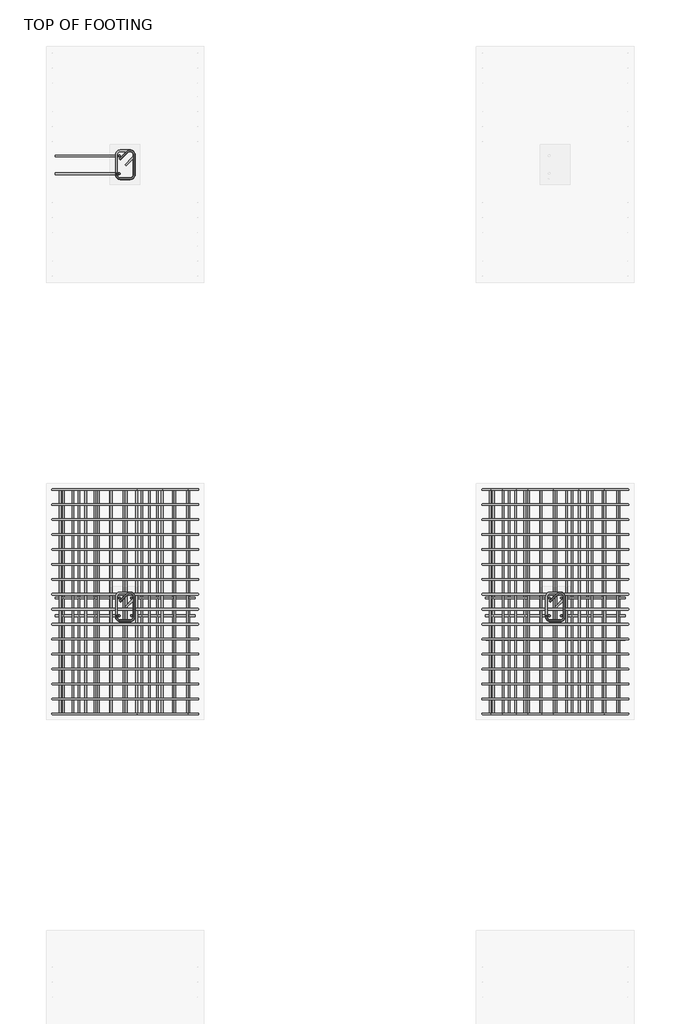
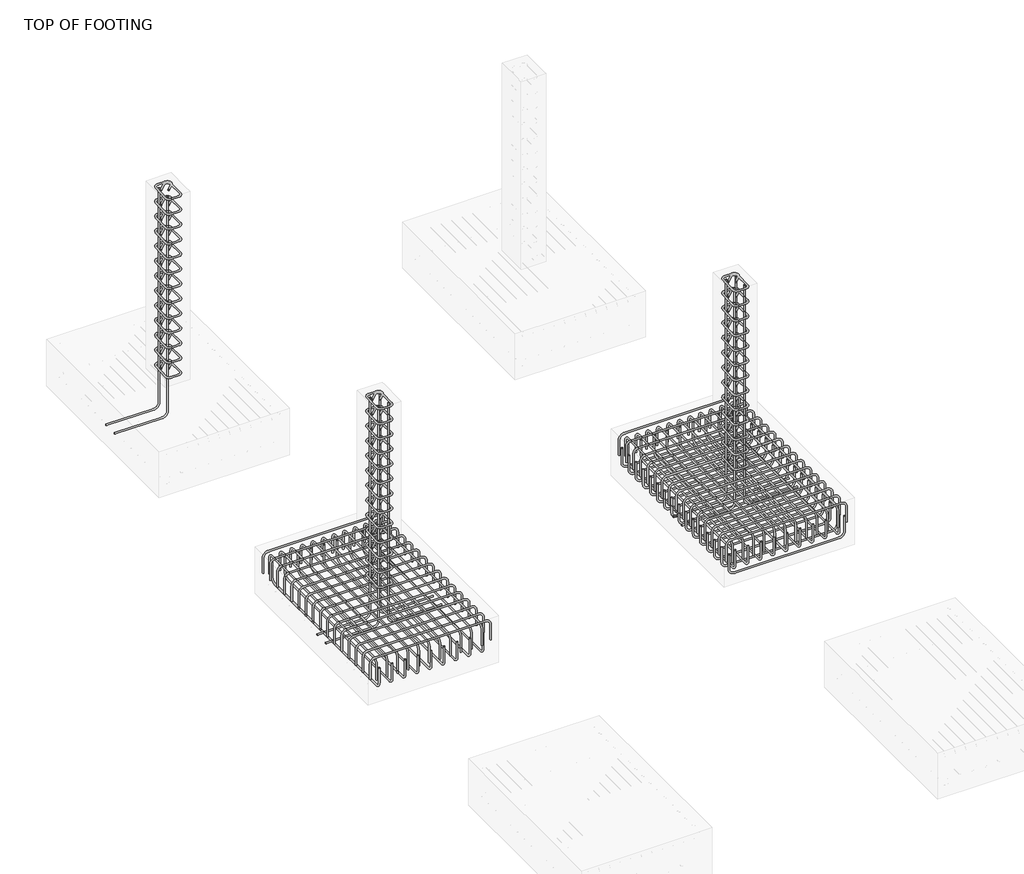
# One storey, part 3 of 8: 15 reinforcing bars.
"""IFC4 building model written with IfcOpenShell, lengths in millimetres."""

from ifc_helpers import new_model, si_unit, point, frame, origin, place, context, project, spatial, polyline, circle_curve, trimmed, segment, composite_curve, source, transform, mapped, element, save
from ifc_brep_helpers import swept_disk

model = new_model("IFC4")

# Units and contexts
model_context = context("Model", 3, world=origin())
ifc_project = project(units=[si_unit("LENGTHUNIT", "METRE", prefix="MILLI")], contexts=[model_context])

# Site, building, storey
site = spatial("IfcSite", under=ifc_project)
building = spatial("IfcBuilding", under=site)
storey = spatial("IfcBuildingStorey", under=building, Name="TOP OF FOOTING", Elevation=-1828.8)

# Reinforcing bars
placement = place(None, origin())
reinforcing_bar_shape = source(origin(), model_context, "Body", "SolidModel", [
    swept_disk(composite_curve([segment(polyline([(-5782.0568817, 6451.7662126, -2068.8), (-5782.0568817, 6451.7662126, -1921.5)]), True, "CONTINUOUS"), segment(trimmed(circle_curve(frame((-5735.7068817, 6451.7662126, -1921.5), z_axis=(0.0, 1.0, 0.0), x_axis=(-46.350000000000364, 0.0, 0.0)), 46.35), [point((-5782.0568817, 6451.7662126, -1921.5))], [point((-5735.7068817, 6451.7662126, -1875.15))], True, "CARTESIAN"), True, "CONTINUOUS"), segment(polyline([(-5735.7068817, 6451.7662126, -1875.15), (-4721.1068817, 6451.7662126, -1875.15)]), True, "CONTINUOUS"), segment(trimmed(circle_curve(frame((-4721.1068817, 6451.7662126, -1921.5), z_axis=(0.0, 1.0, 0.0), x_axis=(0.0, 0.0, 46.34999999999991)), 46.35), [point((-4721.1068817, 6451.7662126, -1875.15))], [point((-4674.7568817, 6451.7662126, -1921.5))], True, "CARTESIAN"), True, "CONTINUOUS"), segment(polyline([(-4674.7568817, 6451.7662126, -1921.5), (-4674.7568817, 6451.7662126, -2068.8)]), True, "CONTINUOUS")], self_intersect=False), 6.35),
])
element("IfcReinforcingBar", 1, at=placement, inside=storey, context=model_context, shape_type="MappedRepresentation", body=[
    mapped(reinforcing_bar_shape, transform((0.0, 0.0, 0.0), x_axis=(1.0, 0.0, 0.0), y_axis=(0.0, 1.0, 0.0), z_axis=(0.0, 0.0, 1.0))),
    mapped(reinforcing_bar_shape, transform((0.0, -113.82, 0.0), x_axis=(1.0, 0.0, 0.0), y_axis=(0.0, 1.0, 0.0), z_axis=(0.0, 0.0, 1.0))),
    mapped(reinforcing_bar_shape, transform((0.0, -227.64, 0.0), x_axis=(1.0, 0.0, 0.0), y_axis=(0.0, 1.0, 0.0), z_axis=(0.0, 0.0, 1.0))),
    mapped(reinforcing_bar_shape, transform((0.0, -341.46, 0.0), x_axis=(1.0, 0.0, 0.0), y_axis=(0.0, 1.0, 0.0), z_axis=(0.0, 0.0, 1.0))),
    mapped(reinforcing_bar_shape, transform((0.0, -455.28, 0.0), x_axis=(1.0, 0.0, 0.0), y_axis=(0.0, 1.0, 0.0), z_axis=(0.0, 0.0, 1.0))),
    mapped(reinforcing_bar_shape, transform((0.0, -569.1, 0.0), x_axis=(1.0, 0.0, 0.0), y_axis=(0.0, 1.0, 0.0), z_axis=(0.0, 0.0, 1.0))),
    mapped(reinforcing_bar_shape, transform((0.0, -682.92, 0.0), x_axis=(1.0, 0.0, 0.0), y_axis=(0.0, 1.0, 0.0), z_axis=(0.0, 0.0, 1.0))),
    mapped(reinforcing_bar_shape, transform((0.0, -796.74, 0.0), x_axis=(1.0, 0.0, 0.0), y_axis=(0.0, 1.0, 0.0), z_axis=(0.0, 0.0, 1.0))),
    mapped(reinforcing_bar_shape, transform((0.0, -910.56, 0.0), x_axis=(1.0, 0.0, 0.0), y_axis=(0.0, 1.0, 0.0), z_axis=(0.0, 0.0, 1.0))),
    mapped(reinforcing_bar_shape, transform((0.0, -1024.38, 0.0), x_axis=(1.0, 0.0, 0.0), y_axis=(0.0, 1.0, 0.0), z_axis=(0.0, 0.0, 1.0))),
    mapped(reinforcing_bar_shape, transform((0.0, -1138.2, 0.0), x_axis=(1.0, 0.0, 0.0), y_axis=(0.0, 1.0, 0.0), z_axis=(0.0, 0.0, 1.0))),
    mapped(reinforcing_bar_shape, transform((0.0, -1252.02, 0.0), x_axis=(1.0, 0.0, 0.0), y_axis=(0.0, 1.0, 0.0), z_axis=(0.0, 0.0, 1.0))),
    mapped(reinforcing_bar_shape, transform((0.0, -1365.84, 0.0), x_axis=(1.0, 0.0, 0.0), y_axis=(0.0, 1.0, 0.0), z_axis=(0.0, 0.0, 1.0))),
    mapped(reinforcing_bar_shape, transform((0.0, -1479.66, 0.0), x_axis=(1.0, 0.0, 0.0), y_axis=(0.0, 1.0, 0.0), z_axis=(0.0, 0.0, 1.0))),
    mapped(reinforcing_bar_shape, transform((0.0, -1593.48, 0.0), x_axis=(1.0, 0.0, 0.0), y_axis=(0.0, 1.0, 0.0), z_axis=(0.0, 0.0, 1.0))),
    mapped(reinforcing_bar_shape, transform((0.0, -1707.3, 0.0), x_axis=(1.0, 0.0, 0.0), y_axis=(0.0, 1.0, 0.0), z_axis=(0.0, 0.0, 1.0))),
])
reinforcing_bar_2_shape = source(origin(), model_context, "Body", "SolidModel", [
    swept_disk(composite_curve([segment(polyline([(-5699.8348303, 6451.7662126, -1986.9111268), (-5699.8348303, 6451.7662126, -2134.2111268)]), True, "CONTINUOUS"), segment(trimmed(circle_curve(frame((-5699.8348303, 6405.4162126, -2134.2111268), z_axis=(-1.0, 0.0, 0.0), x_axis=(0.0, 46.349999999999454, 0.0)), 46.35), [point((-5699.8348303, 6451.7662126, -2134.2111268))], [point((-5699.8348303, 6405.4162126, -2180.5611268))], True, "CARTESIAN"), True, "CONTINUOUS"), segment(polyline([(-5699.8348303, 6405.4162126, -2180.5611268), (-5699.8348303, 4790.8162126, -2180.5611268)]), True, "CONTINUOUS"), segment(trimmed(circle_curve(frame((-5699.8348303, 4790.8162126, -2134.2111268), z_axis=(-1.0, 0.0, 0.0), x_axis=(0.0, 0.0, -46.34999999999991)), 46.35), [point((-5699.8348303, 4790.8162126, -2180.5611268))], [point((-5699.8348303, 4744.4662126, -2134.2111268))], True, "CARTESIAN"), True, "CONTINUOUS"), segment(polyline([(-5699.8348303, 4744.4662126, -2134.2111268), (-5699.8348303, 4744.4662126, -1986.9111268)]), True, "CONTINUOUS")], self_intersect=False), 6.35),
])
element("IfcReinforcingBar", 2, at=placement, inside=storey, context=model_context, shape_type="MappedRepresentation", body=[
    mapped(reinforcing_bar_2_shape, transform((0.0, 0.0, 0.0), x_axis=(1.0, 0.0, 0.0), y_axis=(0.0, 1.0, 0.0), z_axis=(0.0, 0.0, 1.0))),
    mapped(reinforcing_bar_2_shape, transform((119.5564677, 0.0, 0.0), x_axis=(1.0, 0.0, 0.0), y_axis=(0.0, 1.0, 0.0), z_axis=(0.0, 0.0, 1.0))),
    mapped(reinforcing_bar_2_shape, transform((239.1129355, 0.0, 0.0), x_axis=(1.0, 0.0, 0.0), y_axis=(0.0, 1.0, 0.0), z_axis=(0.0, 0.0, 1.0))),
    mapped(reinforcing_bar_2_shape, transform((358.6694032, 0.0, 0.0), x_axis=(1.0, 0.0, 0.0), y_axis=(0.0, 1.0, 0.0), z_axis=(0.0, 0.0, 1.0))),
    mapped(reinforcing_bar_2_shape, transform((478.2258709, 0.0, 0.0), x_axis=(1.0, 0.0, 0.0), y_axis=(0.0, 1.0, 0.0), z_axis=(0.0, 0.0, 1.0))),
    mapped(reinforcing_bar_2_shape, transform((597.7823387, 0.0, 0.0), x_axis=(1.0, 0.0, 0.0), y_axis=(0.0, 1.0, 0.0), z_axis=(0.0, 0.0, 1.0))),
    mapped(reinforcing_bar_2_shape, transform((717.3388064, 0.0, 0.0), x_axis=(1.0, 0.0, 0.0), y_axis=(0.0, 1.0, 0.0), z_axis=(0.0, 0.0, 1.0))),
    mapped(reinforcing_bar_2_shape, transform((836.8952741, 0.0, 0.0), x_axis=(1.0, 0.0, 0.0), y_axis=(0.0, 1.0, 0.0), z_axis=(0.0, 0.0, 1.0))),
    mapped(reinforcing_bar_2_shape, transform((956.4517419, 0.0, 0.0), x_axis=(1.0, 0.0, 0.0), y_axis=(0.0, 1.0, 0.0), z_axis=(0.0, 0.0, 1.0))),
])
reinforcing_bar_3_shape = source(origin(), model_context, "Body", "SolidModel", [
    swept_disk(composite_curve([segment(polyline([(-4754.0668299, 6451.7662126, -2094.8977257), (-4754.0668299, 6451.7662126, -1947.5977257)]), True, "CONTINUOUS"), segment(trimmed(circle_curve(frame((-4754.0668299, 6405.4162126, -1947.5977257), z_axis=(1.0, 0.0, 0.0), x_axis=(0.0, 46.349999999999454, 0.0)), 46.35), [point((-4754.0668299, 6451.7662126, -1947.5977257))], [point((-4754.0668299, 6405.4162126, -1901.2477257))], True, "CARTESIAN"), True, "CONTINUOUS"), segment(polyline([(-4754.0668299, 6405.4162126, -1901.2477257), (-4754.0668299, 4790.8162126, -1901.2477257)]), True, "CONTINUOUS"), segment(trimmed(circle_curve(frame((-4754.0668299, 4790.8162126, -1947.5977257), z_axis=(1.0, 0.0, 0.0), x_axis=(0.0, 0.0, 46.34999999999991)), 46.35), [point((-4754.0668299, 4790.8162126, -1901.2477257))], [point((-4754.0668299, 4744.4662126, -1947.5977257))], True, "CARTESIAN"), True, "CONTINUOUS"), segment(polyline([(-4754.0668299, 4744.4662126, -1947.5977257), (-4754.0668299, 4744.4662126, -2094.8977257)]), True, "CONTINUOUS")], self_intersect=False), 6.35),
])
element("IfcReinforcingBar", 3, at=placement, inside=storey, context=model_context, shape_type="MappedRepresentation", body=[
    mapped(reinforcing_bar_3_shape, transform((0.0, 0.0, 0.0), x_axis=(1.0, 0.0, 0.0), y_axis=(0.0, 1.0, 0.0), z_axis=(0.0, 0.0, 1.0))),
    mapped(reinforcing_bar_3_shape, transform((-97.0050815, 0.0, 0.0), x_axis=(1.0, 0.0, 0.0), y_axis=(0.0, 1.0, 0.0), z_axis=(0.0, 0.0, 1.0))),
    mapped(reinforcing_bar_3_shape, transform((-194.0101631, 0.0, 0.0), x_axis=(1.0, 0.0, 0.0), y_axis=(0.0, 1.0, 0.0), z_axis=(0.0, 0.0, 1.0))),
    mapped(reinforcing_bar_3_shape, transform((-291.0152446, 0.0, 0.0), x_axis=(1.0, 0.0, 0.0), y_axis=(0.0, 1.0, 0.0), z_axis=(0.0, 0.0, 1.0))),
    mapped(reinforcing_bar_3_shape, transform((-388.0203261, 0.0, 0.0), x_axis=(1.0, 0.0, 0.0), y_axis=(0.0, 1.0, 0.0), z_axis=(0.0, 0.0, 1.0))),
    mapped(reinforcing_bar_3_shape, transform((-485.0254076, 0.0, 0.0), x_axis=(1.0, 0.0, 0.0), y_axis=(0.0, 1.0, 0.0), z_axis=(0.0, 0.0, 1.0))),
    mapped(reinforcing_bar_3_shape, transform((-582.0304892, 0.0, 0.0), x_axis=(1.0, 0.0, 0.0), y_axis=(0.0, 1.0, 0.0), z_axis=(0.0, 0.0, 1.0))),
    mapped(reinforcing_bar_3_shape, transform((-679.0355707, 0.0, 0.0), x_axis=(1.0, 0.0, 0.0), y_axis=(0.0, 1.0, 0.0), z_axis=(0.0, 0.0, 1.0))),
    mapped(reinforcing_bar_3_shape, transform((-776.0406522, 0.0, 0.0), x_axis=(1.0, 0.0, 0.0), y_axis=(0.0, 1.0, 0.0), z_axis=(0.0, 0.0, 1.0))),
    mapped(reinforcing_bar_3_shape, transform((-873.0457338, 0.0, 0.0), x_axis=(1.0, 0.0, 0.0), y_axis=(0.0, 1.0, 0.0), z_axis=(0.0, 0.0, 1.0))),
    mapped(reinforcing_bar_3_shape, transform((-970.0508153, 0.0, 0.0), x_axis=(1.0, 0.0, 0.0), y_axis=(0.0, 1.0, 0.0), z_axis=(0.0, 0.0, 1.0))),
])
reinforcing_bar_4_shape = source(origin(), model_context, "Body", "SolidModel", [
    swept_disk(composite_curve([segment(polyline([(-5269.7182423, 5600.7423139, -46.35), (-5213.9746793, 5656.4858768, -46.35)]), True, "CONTINUOUS"), segment(trimmed(circle_curve(frame((-5191.8068817, 5634.3180792, -46.35), z_axis=(0.0, 0.0, -1.0), x_axis=(-22.167797600000085, 22.167797600000085, 0.0)), 31.35), [point((-5213.9746793, 5656.4858768, -46.35))], [point((-5160.4568817, 5634.3180792, -46.35))], True, "CARTESIAN"), True, "CONTINUOUS"), segment(polyline([(-5160.4568817, 5634.3180792, -46.35), (-5160.4568817, 5484.9180792, -46.35)]), True, "CONTINUOUS"), segment(trimmed(circle_curve(frame((-5191.8068817, 5484.9180792, -46.35), z_axis=(0.0, 0.0, -1.0), x_axis=(31.350000000000364, 0.0, 0.0)), 31.35), [point((-5160.4568817, 5484.9180792, -46.35))], [point((-5191.8068817, 5453.5680792, -46.35))], True, "CARTESIAN"), True, "CONTINUOUS"), segment(polyline([(-5191.8068817, 5453.5680792, -46.35), (-5265.0068817, 5453.5680792, -46.35)]), True, "CONTINUOUS"), segment(trimmed(circle_curve(frame((-5265.0068817, 5484.8620303, -44.4761991), z_axis=(0.0, 0.05977036468717588, -0.9982121535551258), x_axis=(0.0, -31.293951099999504, -1.873800899999999)), 31.35), [point((-5265.0068817, 5453.5680792, -46.35))], [point((-5296.3568817, 5484.8620303, -44.4761991))], True, "CARTESIAN"), True, "CONTINUOUS"), segment(polyline([(-5296.3568817, 5484.8620303, -44.4761991), (-5296.3568817, 5634.3741282, -35.5238009)]), True, "CONTINUOUS"), segment(trimmed(circle_curve(frame((-5265.0068817, 5634.3741282, -35.5238009), z_axis=(0.0, 0.05977036468717588, -0.9982121535551258), x_axis=(-31.349999999999454, 0.0, 0.0)), 31.35), [point((-5296.3568817, 5634.3741282, -35.5238009))], [point((-5265.0068817, 5665.6680792, -33.65))], True, "CARTESIAN"), True, "CONTINUOUS"), segment(polyline([(-5265.0068817, 5665.6680792, -33.65), (-5191.8068817, 5665.6680792, -33.65)]), True, "CONTINUOUS"), segment(trimmed(circle_curve(frame((-5191.8068817, 5634.3180792, -33.65), z_axis=(0.0, 0.0, -1.0), x_axis=(0.0, 31.349999999999454, 0.0)), 31.35), [point((-5191.8068817, 5665.6680792, -33.65))], [point((-5169.6390841, 5612.1502816, -33.65))], True, "CARTESIAN"), True, "CONTINUOUS"), segment(polyline([(-5169.6390841, 5612.1502816, -33.65), (-5225.3826471, 5556.4067187, -33.65)]), True, "CONTINUOUS")], self_intersect=False), 6.35),
])
element("IfcReinforcingBar", 4, at=placement, inside=storey, context=model_context, shape_type="MappedRepresentation", body=[
    mapped(reinforcing_bar_4_shape, transform((0.0, 0.0, 0.0), x_axis=(1.0, 0.0, 0.0), y_axis=(0.0, 1.0, 0.0), z_axis=(0.0, 0.0, 1.0))),
    mapped(reinforcing_bar_4_shape, transform((0.0, 0.0, -144.675), x_axis=(1.0, 0.0, 0.0), y_axis=(0.0, 1.0, 0.0), z_axis=(0.0, 0.0, 1.0))),
    mapped(reinforcing_bar_4_shape, transform((0.0, 0.0, -289.35), x_axis=(1.0, 0.0, 0.0), y_axis=(0.0, 1.0, 0.0), z_axis=(0.0, 0.0, 1.0))),
    mapped(reinforcing_bar_4_shape, transform((0.0, 0.0, -434.025), x_axis=(1.0, 0.0, 0.0), y_axis=(0.0, 1.0, 0.0), z_axis=(0.0, 0.0, 1.0))),
    mapped(reinforcing_bar_4_shape, transform((0.0, 0.0, -578.7), x_axis=(1.0, 0.0, 0.0), y_axis=(0.0, 1.0, 0.0), z_axis=(0.0, 0.0, 1.0))),
    mapped(reinforcing_bar_4_shape, transform((0.0, 0.0, -723.375), x_axis=(1.0, 0.0, 0.0), y_axis=(0.0, 1.0, 0.0), z_axis=(0.0, 0.0, 1.0))),
    mapped(reinforcing_bar_4_shape, transform((0.0, 0.0, -868.05), x_axis=(1.0, 0.0, 0.0), y_axis=(0.0, 1.0, 0.0), z_axis=(0.0, 0.0, 1.0))),
    mapped(reinforcing_bar_4_shape, transform((0.0, 0.0, -1012.725), x_axis=(1.0, 0.0, 0.0), y_axis=(0.0, 1.0, 0.0), z_axis=(0.0, 0.0, 1.0))),
    mapped(reinforcing_bar_4_shape, transform((0.0, 0.0, -1157.4), x_axis=(1.0, 0.0, 0.0), y_axis=(0.0, 1.0, 0.0), z_axis=(0.0, 0.0, 1.0))),
    mapped(reinforcing_bar_4_shape, transform((0.0, 0.0, -1302.075), x_axis=(1.0, 0.0, 0.0), y_axis=(0.0, 1.0, 0.0), z_axis=(0.0, 0.0, 1.0))),
    mapped(reinforcing_bar_4_shape, transform((0.0, 0.0, -1446.75), x_axis=(1.0, 0.0, 0.0), y_axis=(0.0, 1.0, 0.0), z_axis=(0.0, 0.0, 1.0))),
    mapped(reinforcing_bar_4_shape, transform((0.0, 0.0, -1591.425), x_axis=(1.0, 0.0, 0.0), y_axis=(0.0, 1.0, 0.0), z_axis=(0.0, 0.0, 1.0))),
    mapped(reinforcing_bar_4_shape, transform((0.0, 0.0, -1736.1), x_axis=(1.0, 0.0, 0.0), y_axis=(0.0, 1.0, 0.0), z_axis=(0.0, 0.0, 1.0))),
])
reinforcing_bar_5_shape = source(origin(), model_context, "Body", "SolidModel", [
    swept_disk(composite_curve([segment(polyline([(-4695.380398, 5491.6680792, -2177.1384798), (-5136.5372203, 5491.6680792, -2177.1384798)]), True, "CONTINUOUS"), segment(trimmed(circle_curve(frame((-5136.5372203, 5491.6680792, -2130.7884798), z_axis=(0.0, 1.0, 0.0), x_axis=(0.0, 0.0, -46.34999999999991)), 46.35), [point((-5136.5372203, 5491.6680792, -2177.1384798))], [point((-5182.8872203, 5491.6680792, -2130.7884798))], True, "CARTESIAN"), True, "CONTINUOUS"), segment(polyline([(-5182.8872203, 5491.6680792, -2130.7884798), (-5182.8872203, 5491.6680792, -40.0)]), True, "CONTINUOUS")], self_intersect=False), 6.35),
])
element("IfcReinforcingBar", 5, at=placement, inside=storey, context=model_context, shape_type="MappedRepresentation", body=[
    mapped(reinforcing_bar_5_shape, transform((0.0, 0.0, 0.0), x_axis=(1.0, 0.0, 0.0), y_axis=(0.0, 1.0, 0.0), z_axis=(0.0, 0.0, 1.0))),
    mapped(reinforcing_bar_5_shape, transform((0.0, 135.9, 0.0), x_axis=(1.0, 0.0, 0.0), y_axis=(0.0, 1.0, 0.0), z_axis=(0.0, 0.0, 1.0))),
])
reinforcing_bar_6_shape = source(origin(), model_context, "Body", "SolidModel", [
    swept_disk(composite_curve([segment(polyline([(-5761.4333654, 5491.6680792, -2177.1384798), (-5320.2765432, 5491.6680792, -2177.1384798)]), True, "CONTINUOUS"), segment(trimmed(circle_curve(frame((-5320.2765432, 5491.6680792, -2130.7884798), z_axis=(0.0, -1.0, 0.0), x_axis=(0.0, 0.0, -46.34999999999991)), 46.35), [point((-5320.2765432, 5491.6680792, -2177.1384798))], [point((-5273.9265432, 5491.6680792, -2130.7884798))], True, "CARTESIAN"), True, "CONTINUOUS"), segment(polyline([(-5273.9265432, 5491.6680792, -2130.7884798), (-5273.9265432, 5491.6680792, -40.0)]), True, "CONTINUOUS")], self_intersect=False), 6.35),
])
element("IfcReinforcingBar", 6, at=placement, inside=storey, context=model_context, shape_type="MappedRepresentation", body=[
    mapped(reinforcing_bar_6_shape, transform((0.0, 0.0, 0.0), x_axis=(1.0, 0.0, 0.0), y_axis=(0.0, 1.0, 0.0), z_axis=(0.0, 0.0, 1.0))),
    mapped(reinforcing_bar_6_shape, transform((0.0, 135.9, 0.0), x_axis=(1.0, 0.0, 0.0), y_axis=(0.0, 1.0, 0.0), z_axis=(0.0, 0.0, 1.0))),
])
reinforcing_bar_7_shape = source(origin(), model_context, "Body", "SolidModel", [
    swept_disk(composite_curve([segment(polyline([(-5269.7182423, 8966.4007933, -46.35), (-5213.9746793, 9022.1443562, -46.35)]), True, "CONTINUOUS"), segment(trimmed(circle_curve(frame((-5191.8068817, 8999.9765586, -46.35), z_axis=(0.0, 0.0, -1.0), x_axis=(-22.167797600000085, 22.167797600000995, 0.0)), 31.35), [point((-5213.9746793, 9022.1443562, -46.35))], [point((-5160.4568817, 8999.9765586, -46.35))], True, "CARTESIAN"), True, "CONTINUOUS"), segment(polyline([(-5160.4568817, 8999.9765586, -46.35), (-5160.4568817, 8850.5765586, -46.35)]), True, "CONTINUOUS"), segment(trimmed(circle_curve(frame((-5191.8068817, 8850.5765586, -46.35), z_axis=(0.0, 0.0, -1.0), x_axis=(31.350000000000364, 0.0, 0.0)), 31.35), [point((-5160.4568817, 8850.5765586, -46.35))], [point((-5191.8068817, 8819.2265586, -46.35))], True, "CARTESIAN"), True, "CONTINUOUS"), segment(polyline([(-5191.8068817, 8819.2265586, -46.35), (-5265.0068817, 8819.2265586, -46.35)]), True, "CONTINUOUS"), segment(trimmed(circle_curve(frame((-5265.0068817, 8850.5205096, -44.4761991), z_axis=(0.0, 0.05977036468717588, -0.9982121535551258), x_axis=(0.0, -31.29395100000147, -1.873800899999999)), 31.35), [point((-5265.0068817, 8819.2265586, -46.35))], [point((-5296.3568817, 8850.5205096, -44.4761991))], True, "CARTESIAN"), True, "CONTINUOUS"), segment(polyline([(-5296.3568817, 8850.5205096, -44.4761991), (-5296.3568817, 9000.0326076, -35.5238009)]), True, "CONTINUOUS"), segment(trimmed(circle_curve(frame((-5265.0068817, 9000.0326076, -35.5238009), z_axis=(0.0, 0.05977036468717588, -0.9982121535551258), x_axis=(-31.349999999999454, 0.0, 0.0)), 31.35), [point((-5296.3568817, 9000.0326076, -35.5238009))], [point((-5265.0068817, 9031.3265586, -33.65))], True, "CARTESIAN"), True, "CONTINUOUS"), segment(polyline([(-5265.0068817, 9031.3265586, -33.65), (-5191.8068817, 9031.3265586, -33.65)]), True, "CONTINUOUS"), segment(trimmed(circle_curve(frame((-5191.8068817, 8999.9765586, -33.65), z_axis=(0.0, 0.0, -1.0), x_axis=(0.0, 31.350000000000364, 0.0)), 31.35), [point((-5191.8068817, 9031.3265586, -33.65))], [point((-5169.6390841, 8977.808761, -33.65))], True, "CARTESIAN"), True, "CONTINUOUS"), segment(polyline([(-5169.6390841, 8977.808761, -33.65), (-5225.3826471, 8922.0651981, -33.65)]), True, "CONTINUOUS")], self_intersect=False), 6.35),
])
element("IfcReinforcingBar", 7, at=placement, inside=storey, context=model_context, shape_type="MappedRepresentation", body=[
    mapped(reinforcing_bar_7_shape, transform((0.0, 0.0, 0.0), x_axis=(1.0, 0.0, 0.0), y_axis=(0.0, 1.0, 0.0), z_axis=(0.0, 0.0, 1.0))),
    mapped(reinforcing_bar_7_shape, transform((0.0, 0.0, -144.675), x_axis=(1.0, 0.0, 0.0), y_axis=(0.0, 1.0, 0.0), z_axis=(0.0, 0.0, 1.0))),
    mapped(reinforcing_bar_7_shape, transform((0.0, 0.0, -289.35), x_axis=(1.0, 0.0, 0.0), y_axis=(0.0, 1.0, 0.0), z_axis=(0.0, 0.0, 1.0))),
    mapped(reinforcing_bar_7_shape, transform((0.0, 0.0, -434.025), x_axis=(1.0, 0.0, 0.0), y_axis=(0.0, 1.0, 0.0), z_axis=(0.0, 0.0, 1.0))),
    mapped(reinforcing_bar_7_shape, transform((0.0, 0.0, -578.7), x_axis=(1.0, 0.0, 0.0), y_axis=(0.0, 1.0, 0.0), z_axis=(0.0, 0.0, 1.0))),
    mapped(reinforcing_bar_7_shape, transform((0.0, 0.0, -723.375), x_axis=(1.0, 0.0, 0.0), y_axis=(0.0, 1.0, 0.0), z_axis=(0.0, 0.0, 1.0))),
    mapped(reinforcing_bar_7_shape, transform((0.0, 0.0, -868.05), x_axis=(1.0, 0.0, 0.0), y_axis=(0.0, 1.0, 0.0), z_axis=(0.0, 0.0, 1.0))),
    mapped(reinforcing_bar_7_shape, transform((0.0, 0.0, -1012.725), x_axis=(1.0, 0.0, 0.0), y_axis=(0.0, 1.0, 0.0), z_axis=(0.0, 0.0, 1.0))),
    mapped(reinforcing_bar_7_shape, transform((0.0, 0.0, -1157.4), x_axis=(1.0, 0.0, 0.0), y_axis=(0.0, 1.0, 0.0), z_axis=(0.0, 0.0, 1.0))),
    mapped(reinforcing_bar_7_shape, transform((0.0, 0.0, -1302.075), x_axis=(1.0, 0.0, 0.0), y_axis=(0.0, 1.0, 0.0), z_axis=(0.0, 0.0, 1.0))),
    mapped(reinforcing_bar_7_shape, transform((0.0, 0.0, -1446.75), x_axis=(1.0, 0.0, 0.0), y_axis=(0.0, 1.0, 0.0), z_axis=(0.0, 0.0, 1.0))),
    mapped(reinforcing_bar_7_shape, transform((0.0, 0.0, -1591.425), x_axis=(1.0, 0.0, 0.0), y_axis=(0.0, 1.0, 0.0), z_axis=(0.0, 0.0, 1.0))),
    mapped(reinforcing_bar_7_shape, transform((0.0, 0.0, -1736.1), x_axis=(1.0, 0.0, 0.0), y_axis=(0.0, 1.0, 0.0), z_axis=(0.0, 0.0, 1.0))),
])
reinforcing_bar_8_shape = source(origin(), model_context, "Body", "SolidModel", [
    swept_disk(composite_curve([segment(polyline([(-5761.4333654, 8857.3265586, -2177.1384798), (-5320.2765432, 8857.3265586, -2177.1384798)]), True, "CONTINUOUS"), segment(trimmed(circle_curve(frame((-5320.2765432, 8857.3265586, -2130.7884798), z_axis=(0.0, -1.0, 0.0), x_axis=(0.0, 0.0, -46.34999999999991)), 46.35), [point((-5320.2765432, 8857.3265586, -2177.1384798))], [point((-5273.9265432, 8857.3265586, -2130.7884798))], True, "CARTESIAN"), True, "CONTINUOUS"), segment(polyline([(-5273.9265432, 8857.3265586, -2130.7884798), (-5273.9265432, 8857.3265586, -40.0)]), True, "CONTINUOUS")], self_intersect=False), 6.35),
])
element("IfcReinforcingBar", 8, at=placement, inside=storey, context=model_context, shape_type="MappedRepresentation", body=[
    mapped(reinforcing_bar_8_shape, transform((0.0, 0.0, 0.0), x_axis=(1.0, 0.0, 0.0), y_axis=(0.0, 1.0, 0.0), z_axis=(0.0, 0.0, 1.0))),
    mapped(reinforcing_bar_8_shape, transform((0.0, 135.9, 0.0), x_axis=(1.0, 0.0, 0.0), y_axis=(0.0, 1.0, 0.0), z_axis=(0.0, 0.0, 1.0))),
])
reinforcing_bar_9_shape = source(origin(), model_context, "Body", "SolidModel", [
    swept_disk(composite_curve([segment(polyline([(-1993.1182423, 5600.7423139, -46.35), (-1937.3746793, 5656.4858768, -46.35)]), True, "CONTINUOUS"), segment(trimmed(circle_curve(frame((-1915.2068817, 5634.3180792, -46.35), z_axis=(0.0, 0.0, -1.0), x_axis=(-22.167797600000085, 22.167797600000085, 0.0)), 31.35), [point((-1937.3746793, 5656.4858768, -46.35))], [point((-1883.8568817, 5634.3180792, -46.35))], True, "CARTESIAN"), True, "CONTINUOUS"), segment(polyline([(-1883.8568817, 5634.3180792, -46.35), (-1883.8568817, 5484.9180792, -46.35)]), True, "CONTINUOUS"), segment(trimmed(circle_curve(frame((-1915.2068817, 5484.9180792, -46.35), z_axis=(0.0, 0.0, -1.0), x_axis=(31.34999999999991, 0.0, 0.0)), 31.35), [point((-1883.8568817, 5484.9180792, -46.35))], [point((-1915.2068817, 5453.5680792, -46.35))], True, "CARTESIAN"), True, "CONTINUOUS"), segment(polyline([(-1915.2068817, 5453.5680792, -46.35), (-1988.4068817, 5453.5680792, -46.35)]), True, "CONTINUOUS"), segment(trimmed(circle_curve(frame((-1988.4068817, 5484.8620303, -44.4761991), z_axis=(0.0, 0.05977036468717588, -0.9982121535551258), x_axis=(0.0, -31.293951099999504, -1.873800899999999)), 31.35), [point((-1988.4068817, 5453.5680792, -46.35))], [point((-2019.7568817, 5484.8620303, -44.4761991))], True, "CARTESIAN"), True, "CONTINUOUS"), segment(polyline([(-2019.7568817, 5484.8620303, -44.4761991), (-2019.7568817, 5634.3741282, -35.5238009)]), True, "CONTINUOUS"), segment(trimmed(circle_curve(frame((-1988.4068817, 5634.3741282, -35.5238009), z_axis=(0.0, 0.05977036468717588, -0.9982121535551258), x_axis=(-31.34999999999991, 0.0, 0.0)), 31.35), [point((-2019.7568817, 5634.3741282, -35.5238009))], [point((-1988.4068817, 5665.6680792, -33.65))], True, "CARTESIAN"), True, "CONTINUOUS"), segment(polyline([(-1988.4068817, 5665.6680792, -33.65), (-1915.2068817, 5665.6680792, -33.65)]), True, "CONTINUOUS"), segment(trimmed(circle_curve(frame((-1915.2068817, 5634.3180792, -33.65), z_axis=(0.0, 0.0, -1.0), x_axis=(0.0, 31.349999999999454, 0.0)), 31.35), [point((-1915.2068817, 5665.6680792, -33.65))], [point((-1893.0390841, 5612.1502816, -33.65))], True, "CARTESIAN"), True, "CONTINUOUS"), segment(polyline([(-1893.0390841, 5612.1502816, -33.65), (-1948.7826471, 5556.4067187, -33.65)]), True, "CONTINUOUS")], self_intersect=False), 6.35),
])
element("IfcReinforcingBar", 9, at=placement, inside=storey, context=model_context, shape_type="MappedRepresentation", body=[
    mapped(reinforcing_bar_9_shape, transform((0.0, 0.0, 0.0), x_axis=(1.0, 0.0, 0.0), y_axis=(0.0, 1.0, 0.0), z_axis=(0.0, 0.0, 1.0))),
    mapped(reinforcing_bar_9_shape, transform((0.0, 0.0, -144.675), x_axis=(1.0, 0.0, 0.0), y_axis=(0.0, 1.0, 0.0), z_axis=(0.0, 0.0, 1.0))),
    mapped(reinforcing_bar_9_shape, transform((0.0, 0.0, -289.35), x_axis=(1.0, 0.0, 0.0), y_axis=(0.0, 1.0, 0.0), z_axis=(0.0, 0.0, 1.0))),
    mapped(reinforcing_bar_9_shape, transform((0.0, 0.0, -434.025), x_axis=(1.0, 0.0, 0.0), y_axis=(0.0, 1.0, 0.0), z_axis=(0.0, 0.0, 1.0))),
    mapped(reinforcing_bar_9_shape, transform((0.0, 0.0, -578.7), x_axis=(1.0, 0.0, 0.0), y_axis=(0.0, 1.0, 0.0), z_axis=(0.0, 0.0, 1.0))),
    mapped(reinforcing_bar_9_shape, transform((0.0, 0.0, -723.375), x_axis=(1.0, 0.0, 0.0), y_axis=(0.0, 1.0, 0.0), z_axis=(0.0, 0.0, 1.0))),
    mapped(reinforcing_bar_9_shape, transform((0.0, 0.0, -868.05), x_axis=(1.0, 0.0, 0.0), y_axis=(0.0, 1.0, 0.0), z_axis=(0.0, 0.0, 1.0))),
    mapped(reinforcing_bar_9_shape, transform((0.0, 0.0, -1012.725), x_axis=(1.0, 0.0, 0.0), y_axis=(0.0, 1.0, 0.0), z_axis=(0.0, 0.0, 1.0))),
    mapped(reinforcing_bar_9_shape, transform((0.0, 0.0, -1157.4), x_axis=(1.0, 0.0, 0.0), y_axis=(0.0, 1.0, 0.0), z_axis=(0.0, 0.0, 1.0))),
    mapped(reinforcing_bar_9_shape, transform((0.0, 0.0, -1302.075), x_axis=(1.0, 0.0, 0.0), y_axis=(0.0, 1.0, 0.0), z_axis=(0.0, 0.0, 1.0))),
    mapped(reinforcing_bar_9_shape, transform((0.0, 0.0, -1446.75), x_axis=(1.0, 0.0, 0.0), y_axis=(0.0, 1.0, 0.0), z_axis=(0.0, 0.0, 1.0))),
    mapped(reinforcing_bar_9_shape, transform((0.0, 0.0, -1591.425), x_axis=(1.0, 0.0, 0.0), y_axis=(0.0, 1.0, 0.0), z_axis=(0.0, 0.0, 1.0))),
    mapped(reinforcing_bar_9_shape, transform((0.0, 0.0, -1736.1), x_axis=(1.0, 0.0, 0.0), y_axis=(0.0, 1.0, 0.0), z_axis=(0.0, 0.0, 1.0))),
])
reinforcing_bar_10_shape = source(origin(), model_context, "Body", "SolidModel", [
    swept_disk(composite_curve([segment(polyline([(-1418.780398, 5491.6680792, -2177.1384798), (-1859.9372203, 5491.6680792, -2177.1384798)]), True, "CONTINUOUS"), segment(trimmed(circle_curve(frame((-1859.9372203, 5491.6680792, -2130.7884798), z_axis=(0.0, 1.0, 0.0), x_axis=(0.0, 0.0, -46.34999999999991)), 46.35), [point((-1859.9372203, 5491.6680792, -2177.1384798))], [point((-1906.2872203, 5491.6680792, -2130.7884798))], True, "CARTESIAN"), True, "CONTINUOUS"), segment(polyline([(-1906.2872203, 5491.6680792, -2130.7884798), (-1906.2872203, 5491.6680792, -40.0)]), True, "CONTINUOUS")], self_intersect=False), 6.35),
])
element("IfcReinforcingBar", 10, at=placement, inside=storey, context=model_context, shape_type="MappedRepresentation", body=[
    mapped(reinforcing_bar_10_shape, transform((0.0, 0.0, 0.0), x_axis=(1.0, 0.0, 0.0), y_axis=(0.0, 1.0, 0.0), z_axis=(0.0, 0.0, 1.0))),
    mapped(reinforcing_bar_10_shape, transform((0.0, 135.9, 0.0), x_axis=(1.0, 0.0, 0.0), y_axis=(0.0, 1.0, 0.0), z_axis=(0.0, 0.0, 1.0))),
])
reinforcing_bar_11_shape = source(origin(), model_context, "Body", "SolidModel", [
    swept_disk(composite_curve([segment(polyline([(-2484.8333654, 5491.6680792, -2177.1384798), (-2043.6765432, 5491.6680792, -2177.1384798)]), True, "CONTINUOUS"), segment(trimmed(circle_curve(frame((-2043.6765432, 5491.6680792, -2130.7884798), z_axis=(0.0, -1.0, 0.0), x_axis=(0.0, 0.0, -46.34999999999991)), 46.35), [point((-2043.6765432, 5491.6680792, -2177.1384798))], [point((-1997.3265432, 5491.6680792, -2130.7884798))], True, "CARTESIAN"), True, "CONTINUOUS"), segment(polyline([(-1997.3265432, 5491.6680792, -2130.7884798), (-1997.3265432, 5491.6680792, -40.0)]), True, "CONTINUOUS")], self_intersect=False), 6.35),
])
element("IfcReinforcingBar", 11, at=placement, inside=storey, context=model_context, shape_type="MappedRepresentation", body=[
    mapped(reinforcing_bar_11_shape, transform((0.0, 0.0, 0.0), x_axis=(1.0, 0.0, 0.0), y_axis=(0.0, 1.0, 0.0), z_axis=(0.0, 0.0, 1.0))),
    mapped(reinforcing_bar_11_shape, transform((0.0, 135.9, 0.0), x_axis=(1.0, 0.0, 0.0), y_axis=(0.0, 1.0, 0.0), z_axis=(0.0, 0.0, 1.0))),
])
reinforcing_bar_12_shape = source(origin(), model_context, "Body", "SolidModel", [
    swept_disk(composite_curve([segment(polyline([(-1417.5573229, 6451.7662126, -2008.2544267), (-1417.5573229, 6451.7662126, -2155.5544267)]), True, "CONTINUOUS"), segment(trimmed(circle_curve(frame((-1463.9073229, 6451.7662126, -2155.5544267), z_axis=(0.0, 1.0, 0.0), x_axis=(46.350000000000136, 0.0, 0.0)), 46.35), [point((-1417.5573229, 6451.7662126, -2155.5544267))], [point((-1463.9073229, 6451.7662126, -2201.9044267))], True, "CARTESIAN"), True, "CONTINUOUS"), segment(polyline([(-1463.9073229, 6451.7662126, -2201.9044267), (-2434.9233592, 6451.7662126, -2201.9044267)]), True, "CONTINUOUS"), segment(trimmed(circle_curve(frame((-2434.9233592, 6451.7662126, -2155.5544267), z_axis=(0.0, 1.0, 0.0), x_axis=(0.0, 0.0, -46.34999999999991)), 46.35), [point((-2434.9233592, 6451.7662126, -2201.9044267))], [point((-2481.2733592, 6451.7662126, -2155.5544267))], True, "CARTESIAN"), True, "CONTINUOUS"), segment(polyline([(-2481.2733592, 6451.7662126, -2155.5544267), (-2481.2733592, 6451.7662126, -2008.2544267)]), True, "CONTINUOUS")], self_intersect=False), 6.35),
])
element("IfcReinforcingBar", 12, at=placement, inside=storey, context=model_context, shape_type="MappedRepresentation", body=[
    mapped(reinforcing_bar_12_shape, transform((0.0, 0.0, 0.0), x_axis=(1.0, 0.0, 0.0), y_axis=(0.0, 1.0, 0.0), z_axis=(0.0, 0.0, 1.0))),
    mapped(reinforcing_bar_12_shape, transform((0.0, -113.82, 0.0), x_axis=(1.0, 0.0, 0.0), y_axis=(0.0, 1.0, 0.0), z_axis=(0.0, 0.0, 1.0))),
    mapped(reinforcing_bar_12_shape, transform((0.0, -227.64, 0.0), x_axis=(1.0, 0.0, 0.0), y_axis=(0.0, 1.0, 0.0), z_axis=(0.0, 0.0, 1.0))),
    mapped(reinforcing_bar_12_shape, transform((0.0, -341.46, 0.0), x_axis=(1.0, 0.0, 0.0), y_axis=(0.0, 1.0, 0.0), z_axis=(0.0, 0.0, 1.0))),
    mapped(reinforcing_bar_12_shape, transform((0.0, -455.28, 0.0), x_axis=(1.0, 0.0, 0.0), y_axis=(0.0, 1.0, 0.0), z_axis=(0.0, 0.0, 1.0))),
    mapped(reinforcing_bar_12_shape, transform((0.0, -569.1, 0.0), x_axis=(1.0, 0.0, 0.0), y_axis=(0.0, 1.0, 0.0), z_axis=(0.0, 0.0, 1.0))),
    mapped(reinforcing_bar_12_shape, transform((0.0, -682.92, 0.0), x_axis=(1.0, 0.0, 0.0), y_axis=(0.0, 1.0, 0.0), z_axis=(0.0, 0.0, 1.0))),
    mapped(reinforcing_bar_12_shape, transform((0.0, -796.74, 0.0), x_axis=(1.0, 0.0, 0.0), y_axis=(0.0, 1.0, 0.0), z_axis=(0.0, 0.0, 1.0))),
    mapped(reinforcing_bar_12_shape, transform((0.0, -910.56, 0.0), x_axis=(1.0, 0.0, 0.0), y_axis=(0.0, 1.0, 0.0), z_axis=(0.0, 0.0, 1.0))),
    mapped(reinforcing_bar_12_shape, transform((0.0, -1024.38, 0.0), x_axis=(1.0, 0.0, 0.0), y_axis=(0.0, 1.0, 0.0), z_axis=(0.0, 0.0, 1.0))),
    mapped(reinforcing_bar_12_shape, transform((0.0, -1138.2, 0.0), x_axis=(1.0, 0.0, 0.0), y_axis=(0.0, 1.0, 0.0), z_axis=(0.0, 0.0, 1.0))),
    mapped(reinforcing_bar_12_shape, transform((0.0, -1252.02, 0.0), x_axis=(1.0, 0.0, 0.0), y_axis=(0.0, 1.0, 0.0), z_axis=(0.0, 0.0, 1.0))),
    mapped(reinforcing_bar_12_shape, transform((0.0, -1365.84, 0.0), x_axis=(1.0, 0.0, 0.0), y_axis=(0.0, 1.0, 0.0), z_axis=(0.0, 0.0, 1.0))),
    mapped(reinforcing_bar_12_shape, transform((0.0, -1479.66, 0.0), x_axis=(1.0, 0.0, 0.0), y_axis=(0.0, 1.0, 0.0), z_axis=(0.0, 0.0, 1.0))),
    mapped(reinforcing_bar_12_shape, transform((0.0, -1593.48, 0.0), x_axis=(1.0, 0.0, 0.0), y_axis=(0.0, 1.0, 0.0), z_axis=(0.0, 0.0, 1.0))),
    mapped(reinforcing_bar_12_shape, transform((0.0, -1707.3, 0.0), x_axis=(1.0, 0.0, 0.0), y_axis=(0.0, 1.0, 0.0), z_axis=(0.0, 0.0, 1.0))),
])
reinforcing_bar_13_shape = source(origin(), model_context, "Body", "SolidModel", [
    swept_disk(composite_curve([segment(polyline([(-2505.4568817, 6451.7662126, -2068.8), (-2505.4568817, 6451.7662126, -1921.5)]), True, "CONTINUOUS"), segment(trimmed(circle_curve(frame((-2459.1068817, 6451.7662126, -1921.5), z_axis=(0.0, 1.0, 0.0), x_axis=(-46.34999999999991, 0.0, 0.0)), 46.35), [point((-2505.4568817, 6451.7662126, -1921.5))], [point((-2459.1068817, 6451.7662126, -1875.15))], True, "CARTESIAN"), True, "CONTINUOUS"), segment(polyline([(-2459.1068817, 6451.7662126, -1875.15), (-1444.5068817, 6451.7662126, -1875.15)]), True, "CONTINUOUS"), segment(trimmed(circle_curve(frame((-1444.5068817, 6451.7662126, -1921.5), z_axis=(0.0, 1.0, 0.0), x_axis=(0.0, 0.0, 46.34999999999991)), 46.35), [point((-1444.5068817, 6451.7662126, -1875.15))], [point((-1398.1568817, 6451.7662126, -1921.5))], True, "CARTESIAN"), True, "CONTINUOUS"), segment(polyline([(-1398.1568817, 6451.7662126, -1921.5), (-1398.1568817, 6451.7662126, -2068.8)]), True, "CONTINUOUS")], self_intersect=False), 6.35),
])
element("IfcReinforcingBar", 13, at=placement, inside=storey, context=model_context, shape_type="MappedRepresentation", body=[
    mapped(reinforcing_bar_13_shape, transform((0.0, 0.0, 0.0), x_axis=(1.0, 0.0, 0.0), y_axis=(0.0, 1.0, 0.0), z_axis=(0.0, 0.0, 1.0))),
    mapped(reinforcing_bar_13_shape, transform((0.0, -113.82, 0.0), x_axis=(1.0, 0.0, 0.0), y_axis=(0.0, 1.0, 0.0), z_axis=(0.0, 0.0, 1.0))),
    mapped(reinforcing_bar_13_shape, transform((0.0, -227.64, 0.0), x_axis=(1.0, 0.0, 0.0), y_axis=(0.0, 1.0, 0.0), z_axis=(0.0, 0.0, 1.0))),
    mapped(reinforcing_bar_13_shape, transform((0.0, -341.46, 0.0), x_axis=(1.0, 0.0, 0.0), y_axis=(0.0, 1.0, 0.0), z_axis=(0.0, 0.0, 1.0))),
    mapped(reinforcing_bar_13_shape, transform((0.0, -455.28, 0.0), x_axis=(1.0, 0.0, 0.0), y_axis=(0.0, 1.0, 0.0), z_axis=(0.0, 0.0, 1.0))),
    mapped(reinforcing_bar_13_shape, transform((0.0, -569.1, 0.0), x_axis=(1.0, 0.0, 0.0), y_axis=(0.0, 1.0, 0.0), z_axis=(0.0, 0.0, 1.0))),
    mapped(reinforcing_bar_13_shape, transform((0.0, -682.92, 0.0), x_axis=(1.0, 0.0, 0.0), y_axis=(0.0, 1.0, 0.0), z_axis=(0.0, 0.0, 1.0))),
    mapped(reinforcing_bar_13_shape, transform((0.0, -796.74, 0.0), x_axis=(1.0, 0.0, 0.0), y_axis=(0.0, 1.0, 0.0), z_axis=(0.0, 0.0, 1.0))),
    mapped(reinforcing_bar_13_shape, transform((0.0, -910.56, 0.0), x_axis=(1.0, 0.0, 0.0), y_axis=(0.0, 1.0, 0.0), z_axis=(0.0, 0.0, 1.0))),
    mapped(reinforcing_bar_13_shape, transform((0.0, -1024.38, 0.0), x_axis=(1.0, 0.0, 0.0), y_axis=(0.0, 1.0, 0.0), z_axis=(0.0, 0.0, 1.0))),
    mapped(reinforcing_bar_13_shape, transform((0.0, -1138.2, 0.0), x_axis=(1.0, 0.0, 0.0), y_axis=(0.0, 1.0, 0.0), z_axis=(0.0, 0.0, 1.0))),
    mapped(reinforcing_bar_13_shape, transform((0.0, -1252.02, 0.0), x_axis=(1.0, 0.0, 0.0), y_axis=(0.0, 1.0, 0.0), z_axis=(0.0, 0.0, 1.0))),
    mapped(reinforcing_bar_13_shape, transform((0.0, -1365.84, 0.0), x_axis=(1.0, 0.0, 0.0), y_axis=(0.0, 1.0, 0.0), z_axis=(0.0, 0.0, 1.0))),
    mapped(reinforcing_bar_13_shape, transform((0.0, -1479.66, 0.0), x_axis=(1.0, 0.0, 0.0), y_axis=(0.0, 1.0, 0.0), z_axis=(0.0, 0.0, 1.0))),
    mapped(reinforcing_bar_13_shape, transform((0.0, -1593.48, 0.0), x_axis=(1.0, 0.0, 0.0), y_axis=(0.0, 1.0, 0.0), z_axis=(0.0, 0.0, 1.0))),
    mapped(reinforcing_bar_13_shape, transform((0.0, -1707.3, 0.0), x_axis=(1.0, 0.0, 0.0), y_axis=(0.0, 1.0, 0.0), z_axis=(0.0, 0.0, 1.0))),
])
reinforcing_bar_14_shape = source(origin(), model_context, "Body", "SolidModel", [
    swept_disk(composite_curve([segment(polyline([(-2423.2348303, 6451.7662126, -1986.9111268), (-2423.2348303, 6451.7662126, -2134.2111268)]), True, "CONTINUOUS"), segment(trimmed(circle_curve(frame((-2423.2348303, 6405.4162126, -2134.2111268), z_axis=(-1.0, 0.0, 0.0), x_axis=(0.0, 46.349999999999454, 0.0)), 46.35), [point((-2423.2348303, 6451.7662126, -2134.2111268))], [point((-2423.2348303, 6405.4162126, -2180.5611268))], True, "CARTESIAN"), True, "CONTINUOUS"), segment(polyline([(-2423.2348303, 6405.4162126, -2180.5611268), (-2423.2348303, 4790.8162126, -2180.5611268)]), True, "CONTINUOUS"), segment(trimmed(circle_curve(frame((-2423.2348303, 4790.8162126, -2134.2111268), z_axis=(-1.0, 0.0, 0.0), x_axis=(0.0, 0.0, -46.34999999999991)), 46.35), [point((-2423.2348303, 4790.8162126, -2180.5611268))], [point((-2423.2348303, 4744.4662126, -2134.2111268))], True, "CARTESIAN"), True, "CONTINUOUS"), segment(polyline([(-2423.2348303, 4744.4662126, -2134.2111268), (-2423.2348303, 4744.4662126, -1986.9111268)]), True, "CONTINUOUS")], self_intersect=False), 6.35),
])
element("IfcReinforcingBar", 14, at=placement, inside=storey, context=model_context, shape_type="MappedRepresentation", body=[
    mapped(reinforcing_bar_14_shape, transform((0.0, 0.0, 0.0), x_axis=(1.0, 0.0, 0.0), y_axis=(0.0, 1.0, 0.0), z_axis=(0.0, 0.0, 1.0))),
    mapped(reinforcing_bar_14_shape, transform((119.5564677, 0.0, 0.0), x_axis=(1.0, 0.0, 0.0), y_axis=(0.0, 1.0, 0.0), z_axis=(0.0, 0.0, 1.0))),
    mapped(reinforcing_bar_14_shape, transform((239.1129355, 0.0, 0.0), x_axis=(1.0, 0.0, 0.0), y_axis=(0.0, 1.0, 0.0), z_axis=(0.0, 0.0, 1.0))),
    mapped(reinforcing_bar_14_shape, transform((358.6694032, 0.0, 0.0), x_axis=(1.0, 0.0, 0.0), y_axis=(0.0, 1.0, 0.0), z_axis=(0.0, 0.0, 1.0))),
    mapped(reinforcing_bar_14_shape, transform((478.2258709, 0.0, 0.0), x_axis=(1.0, 0.0, 0.0), y_axis=(0.0, 1.0, 0.0), z_axis=(0.0, 0.0, 1.0))),
    mapped(reinforcing_bar_14_shape, transform((597.7823387, 0.0, 0.0), x_axis=(1.0, 0.0, 0.0), y_axis=(0.0, 1.0, 0.0), z_axis=(0.0, 0.0, 1.0))),
    mapped(reinforcing_bar_14_shape, transform((717.3388064, 0.0, 0.0), x_axis=(1.0, 0.0, 0.0), y_axis=(0.0, 1.0, 0.0), z_axis=(0.0, 0.0, 1.0))),
    mapped(reinforcing_bar_14_shape, transform((836.8952741, 0.0, 0.0), x_axis=(1.0, 0.0, 0.0), y_axis=(0.0, 1.0, 0.0), z_axis=(0.0, 0.0, 1.0))),
    mapped(reinforcing_bar_14_shape, transform((956.4517419, 0.0, 0.0), x_axis=(1.0, 0.0, 0.0), y_axis=(0.0, 1.0, 0.0), z_axis=(0.0, 0.0, 1.0))),
])
reinforcing_bar_15_shape = source(origin(), model_context, "Body", "SolidModel", [
    swept_disk(composite_curve([segment(polyline([(-1477.4668299, 6451.7662126, -2094.8977257), (-1477.4668299, 6451.7662126, -1947.5977257)]), True, "CONTINUOUS"), segment(trimmed(circle_curve(frame((-1477.4668299, 6405.4162126, -1947.5977257), z_axis=(1.0, 0.0, 0.0), x_axis=(0.0, 46.349999999999454, 0.0)), 46.35), [point((-1477.4668299, 6451.7662126, -1947.5977257))], [point((-1477.4668299, 6405.4162126, -1901.2477257))], True, "CARTESIAN"), True, "CONTINUOUS"), segment(polyline([(-1477.4668299, 6405.4162126, -1901.2477257), (-1477.4668299, 4790.8162126, -1901.2477257)]), True, "CONTINUOUS"), segment(trimmed(circle_curve(frame((-1477.4668299, 4790.8162126, -1947.5977257), z_axis=(1.0, 0.0, 0.0), x_axis=(0.0, 0.0, 46.34999999999991)), 46.35), [point((-1477.4668299, 4790.8162126, -1901.2477257))], [point((-1477.4668299, 4744.4662126, -1947.5977257))], True, "CARTESIAN"), True, "CONTINUOUS"), segment(polyline([(-1477.4668299, 4744.4662126, -1947.5977257), (-1477.4668299, 4744.4662126, -2094.8977257)]), True, "CONTINUOUS")], self_intersect=False), 6.35),
])
element("IfcReinforcingBar", 15, at=placement, inside=storey, context=model_context, shape_type="MappedRepresentation", body=[
    mapped(reinforcing_bar_15_shape, transform((0.0, 0.0, 0.0), x_axis=(1.0, 0.0, 0.0), y_axis=(0.0, 1.0, 0.0), z_axis=(0.0, 0.0, 1.0))),
    mapped(reinforcing_bar_15_shape, transform((-97.0050815, 0.0, 0.0), x_axis=(1.0, 0.0, 0.0), y_axis=(0.0, 1.0, 0.0), z_axis=(0.0, 0.0, 1.0))),
    mapped(reinforcing_bar_15_shape, transform((-194.0101631, 0.0, 0.0), x_axis=(1.0, 0.0, 0.0), y_axis=(0.0, 1.0, 0.0), z_axis=(0.0, 0.0, 1.0))),
    mapped(reinforcing_bar_15_shape, transform((-291.0152446, 0.0, 0.0), x_axis=(1.0, 0.0, 0.0), y_axis=(0.0, 1.0, 0.0), z_axis=(0.0, 0.0, 1.0))),
    mapped(reinforcing_bar_15_shape, transform((-388.0203261, 0.0, 0.0), x_axis=(1.0, 0.0, 0.0), y_axis=(0.0, 1.0, 0.0), z_axis=(0.0, 0.0, 1.0))),
    mapped(reinforcing_bar_15_shape, transform((-485.0254076, 0.0, 0.0), x_axis=(1.0, 0.0, 0.0), y_axis=(0.0, 1.0, 0.0), z_axis=(0.0, 0.0, 1.0))),
    mapped(reinforcing_bar_15_shape, transform((-582.0304892, 0.0, 0.0), x_axis=(1.0, 0.0, 0.0), y_axis=(0.0, 1.0, 0.0), z_axis=(0.0, 0.0, 1.0))),
    mapped(reinforcing_bar_15_shape, transform((-679.0355707, 0.0, 0.0), x_axis=(1.0, 0.0, 0.0), y_axis=(0.0, 1.0, 0.0), z_axis=(0.0, 0.0, 1.0))),
    mapped(reinforcing_bar_15_shape, transform((-776.0406522, 0.0, 0.0), x_axis=(1.0, 0.0, 0.0), y_axis=(0.0, 1.0, 0.0), z_axis=(0.0, 0.0, 1.0))),
    mapped(reinforcing_bar_15_shape, transform((-873.0457338, 0.0, 0.0), x_axis=(1.0, 0.0, 0.0), y_axis=(0.0, 1.0, 0.0), z_axis=(0.0, 0.0, 1.0))),
    mapped(reinforcing_bar_15_shape, transform((-970.0508153, 0.0, 0.0), x_axis=(1.0, 0.0, 0.0), y_axis=(0.0, 1.0, 0.0), z_axis=(0.0, 0.0, 1.0))),
])

save(model, "model.ifc")

# Revit data of these elements
# Elements 1, 2, 3, 4, 5, 6, 7, 8, 9, 10, 11, 12, 13, 14, 15 (IfcReinforcingBar)
#   Phase Created = New Construction
